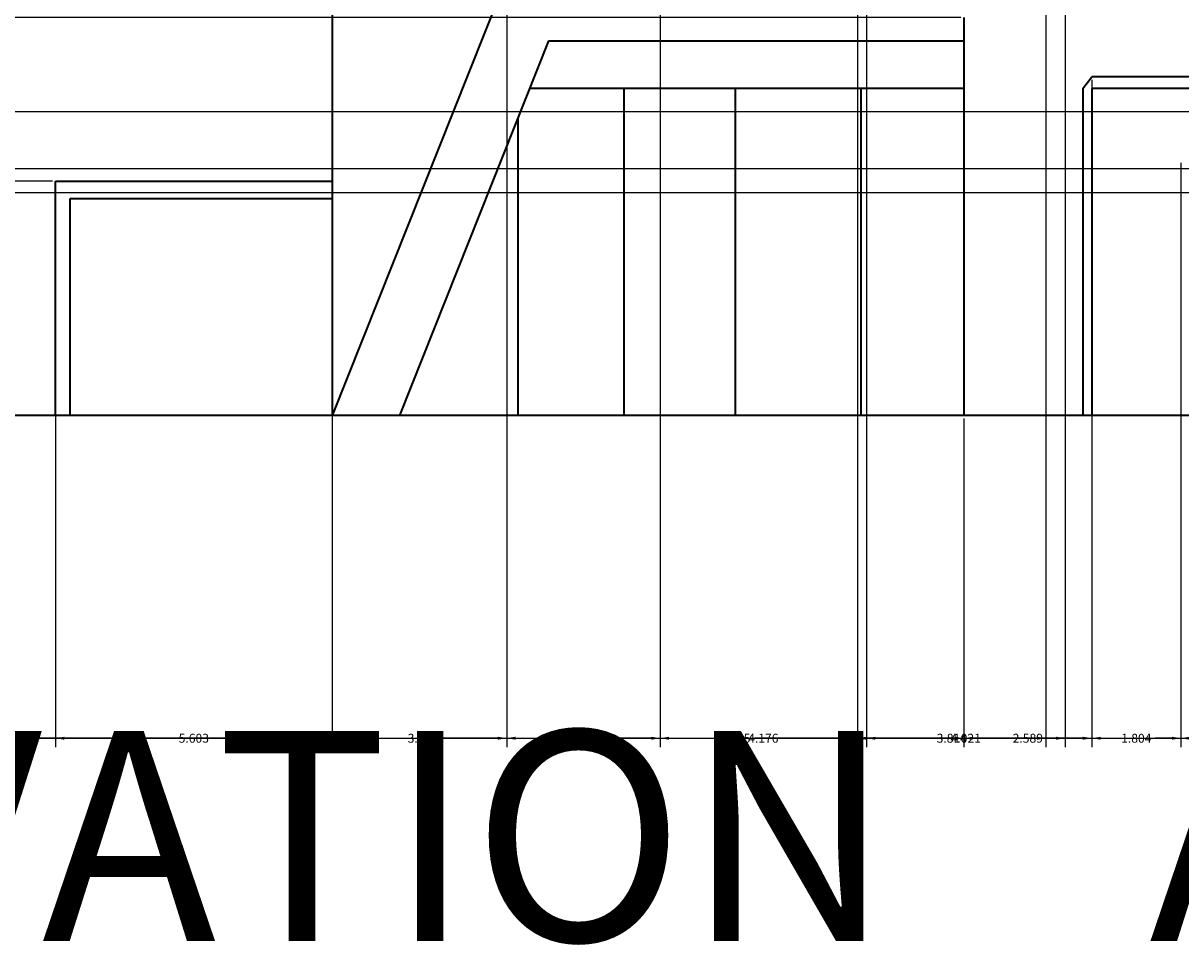
# Model space of a CAD drawing. Units: inches. Extents: x -10 to 130, y -32 to 34.
# Tile 3 of 22: x 25.72 to 49.15, y -32.13 to -13.47. Entities that reach past the tile are written whole.
import ezdxf

# ---------------------------------------------------------------- set-up
doc = ezdxf.new("R2010")
doc.units = ezdxf.units.IN
doc.header["$MEASUREMENT"] = 0
for name, color, linetype, lineweight in [('A-ANNO-DIMS', 2, 'Continuous', 18), ('A-ANNO-TEXT', 7, 'Continuous', 25), ('A-ELEV', 7, 'Continuous', 35)]:
    doc.layers.add(name, color=color, linetype=linetype, lineweight=lineweight)
doc.styles.get("Standard").update_dxf_attribs({"font": 'arial.ttf'})
doc.dimstyles.get("Standard").update_dxf_attribs({"dimtxt": 0.18, "dimasz": 0.18, "dimexe": 0.18, "dimexo": 0.0625, "dimgap": 0.09, "dimtad": 0, "dimtih": 1, "dimtoh": 1, "dimdec": 4, "dimzin": 0, "dimdsep": 46, "dimtxsty": 'Standard', "dimcen": 0.09, "dimadec": 0, "dimazin": 0, "dimtfac": 1, "dimtdec": 4, "dimtofl": 0, "dimtmove": 0, "dimatfit": 3, "dimfxl": 1, "dimtolj": 1, "dimtzin": 0, "dimarcsym": 0})

# ---------------------------------------------------------------- blocks, each defined once
blk = doc.blocks.new('*D1')
at = {"layer": 'A-ANNO-DIMS', "color": 0, "lineweight": -2, "transparency": 16777216}
for p, q in [((5.634, -13.647), (5.634, -28.129)), ((107.933, -21.477), (107.933, -28.129)), ((5.814, -27.949), (56.398, -27.949)), ((107.753, -27.949), (57.169, -27.949))]:
    blk.add_line(p, q, dxfattribs=at)
at = {"layer": 'A-ANNO-DIMS', "color": 0, "transparency": 16777216}
for points in [[(5.814, -27.919), (5.814, -27.979), (5.634, -27.949)], [(107.753, -27.919), (107.753, -27.979), (107.933, -27.949)]]:
    blk.add_solid(points, dxfattribs=at)
at = {"layer": 'Defpoints', "color": 0, "transparency": 16777216}
for p in [(5.634, -13.584), (107.933, -21.414), (107.933, -27.949)]:
    blk.add_point(p, dxfattribs=at)
at = {"layer": 'A-ANNO-DIMS', "color": 0, "transparency": 16777216, "insert": (56.784, -27.949), "char_height": 0.18, "attachment_point": 5}
blk.add_mtext('\\A1;102.3', dxfattribs=at)
blk = doc.blocks.new('*D42')
at = {"layer": 'A-ANNO-DIMS', "color": 0, "lineweight": -2, "transparency": 16777216}
for p, q in [((19.055, -21.477), (19.055, -28.129)), ((31.971, -21.477), (31.971, -28.129)), ((19.235, -27.949), (25.058, -27.949)), ((31.791, -27.949), (25.968, -27.949))]:
    blk.add_line(p, q, dxfattribs=at)
at = {"layer": 'A-ANNO-DIMS', "color": 0, "transparency": 16777216}
for points in [[(19.235, -27.919), (19.235, -27.979), (19.055, -27.949)], [(31.791, -27.919), (31.791, -27.979), (31.971, -27.949)]]:
    blk.add_solid(points, dxfattribs=at)
at = {"layer": 'Defpoints', "color": 0, "transparency": 16777216}
for p in [(19.055, -21.414), (31.971, -21.414), (31.971, -27.949)]:
    blk.add_point(p, dxfattribs=at)
at = {"layer": 'A-ANNO-DIMS', "color": 0, "transparency": 16777216, "insert": (25.513, -27.949), "char_height": 0.18, "attachment_point": 5}
blk.add_mtext('\\A1;12.916', dxfattribs=at)
blk = doc.blocks.new('*D43')
at = {"layer": 'A-ANNO-DIMS', "color": 0, "lineweight": -2, "transparency": 16777216}
for p, q in [((35.505, -12.596), (35.505, -28.129)), ((31.971, -21.477), (31.971, -28.129)), ((32.151, -27.949), (33.414, -27.949)), ((35.325, -27.949), (34.062, -27.949))]:
    blk.add_line(p, q, dxfattribs=at)
at = {"layer": 'A-ANNO-DIMS', "color": 0, "transparency": 16777216}
for points in [[(32.151, -27.919), (32.151, -27.979), (31.971, -27.949)], [(35.325, -27.919), (35.325, -27.979), (35.505, -27.949)]]:
    blk.add_solid(points, dxfattribs=at)
at = {"layer": 'Defpoints', "color": 0, "transparency": 16777216}
for p in [(35.505, -12.534), (31.971, -21.414), (35.505, -27.949)]:
    blk.add_point(p, dxfattribs=at)
at = {"layer": 'A-ANNO-DIMS', "color": 0, "transparency": 16777216, "insert": (33.738, -27.949), "char_height": 0.18, "attachment_point": 5}
blk.add_mtext('\\A1;3.53', dxfattribs=at)
blk = doc.blocks.new('*D44')
at = {"layer": 'A-ANNO-DIMS', "color": 0, "lineweight": -2, "transparency": 16777216}
for p, q in [((35.505, -12.596), (35.505, -28.129)), ((44.76, -21.477), (44.76, -28.129)), ((35.685, -27.949), (39.738, -27.949)), ((44.58, -27.949), (40.527, -27.949))]:
    blk.add_line(p, q, dxfattribs=at)
at = {"layer": 'A-ANNO-DIMS', "color": 0, "transparency": 16777216}
for points in [[(35.685, -27.919), (35.685, -27.979), (35.505, -27.949)], [(44.58, -27.919), (44.58, -27.979), (44.76, -27.949)]]:
    blk.add_solid(points, dxfattribs=at)
at = {"layer": 'Defpoints', "color": 0, "transparency": 16777216}
for p in [(35.505, -12.534), (44.76, -21.414), (44.76, -27.949)]:
    blk.add_point(p, dxfattribs=at)
at = {"layer": 'A-ANNO-DIMS', "color": 0, "transparency": 16777216, "insert": (40.132, -27.949), "char_height": 0.18, "attachment_point": 5}
blk.add_mtext('\\A1;9.255', dxfattribs=at)
blk = doc.blocks.new('*D47')
at = {"layer": 'A-ANNO-DIMS', "color": 0, "lineweight": -2, "transparency": 16777216}
for p, q in [((35.567, -12.534), (129.508, -12.534)), ((129.328, -12.714), (129.328, -16.792)), ((129.328, -21.234), (129.328, -17.156)), ((32.034, -21.414), (129.508, -21.414))]:
    blk.add_line(p, q, dxfattribs=at)
at = {"layer": 'A-ANNO-DIMS', "color": 0, "transparency": 16777216}
for points in [[(129.298, -12.714), (129.358, -12.714), (129.328, -12.534)], [(129.298, -21.234), (129.358, -21.234), (129.328, -21.414)]]:
    blk.add_solid(points, dxfattribs=at)
at = {"layer": 'Defpoints', "color": 0, "transparency": 16777216}
for p in [(35.505, -12.534), (31.971, -21.414), (129.328, -21.414)]:
    blk.add_point(p, dxfattribs=at)
at = {"layer": 'A-ANNO-DIMS', "color": 0, "transparency": 16777216, "insert": (129.328, -16.974), "char_height": 0.18, "attachment_point": 5}
blk.add_mtext('\\A1;8.88', dxfattribs=at)
blk = doc.blocks.new('*D49')
at = {"layer": 'A-ANNO-DIMS', "color": 0, "lineweight": -2, "transparency": 16777216}
for p, q in [((44.697, -13.356), (-9.564, -13.356)), ((-9.384, -13.536), (-9.384, -17.203)), ((-9.384, -21.234), (-9.384, -17.567)), ((44.697, -21.414), (-9.564, -21.414))]:
    blk.add_line(p, q, dxfattribs=at)
at = {"layer": 'A-ANNO-DIMS', "color": 0, "transparency": 16777216}
for points in [[(-9.414, -13.536), (-9.354, -13.536), (-9.384, -13.356)], [(-9.414, -21.234), (-9.354, -21.234), (-9.384, -21.414)]]:
    blk.add_solid(points, dxfattribs=at)
at = {"layer": 'Defpoints', "color": 0, "transparency": 16777216}
for p in [(44.76, -13.356), (-9.384, -21.414), (44.76, -21.414)]:
    blk.add_point(p, dxfattribs=at)
at = {"layer": 'A-ANNO-DIMS', "color": 0, "transparency": 16777216, "insert": (-9.384, -17.385), "char_height": 0.18, "attachment_point": 5}
blk.add_mtext('\\A1;8.059', dxfattribs=at)
blk = doc.blocks.new('*D50')
at = {"layer": 'A-ANNO-DIMS', "color": 0, "lineweight": -2, "transparency": 16777216}
for p, q in [((47.349, -14.617), (47.349, -28.129)), ((44.76, -21.477), (44.76, -28.129)), ((44.94, -27.949), (45.659, -27.949)), ((47.169, -27.949), (46.45, -27.949))]:
    blk.add_line(p, q, dxfattribs=at)
at = {"layer": 'A-ANNO-DIMS', "color": 0, "transparency": 16777216}
for points in [[(44.94, -27.919), (44.94, -27.979), (44.76, -27.949)], [(47.169, -27.919), (47.169, -27.979), (47.349, -27.949)]]:
    blk.add_solid(points, dxfattribs=at)
at = {"layer": 'Defpoints', "color": 0, "transparency": 16777216}
for p in [(47.349, -14.555), (44.76, -21.414), (47.349, -27.949)]:
    blk.add_point(p, dxfattribs=at)
at = {"layer": 'A-ANNO-DIMS', "color": 0, "transparency": 16777216, "insert": (46.055, -27.949), "char_height": 0.18, "attachment_point": 5}
blk.add_mtext('\\A1;2.589', dxfattribs=at)
blk = doc.blocks.new('*D51')
at = {"layer": 'A-ANNO-DIMS', "color": 0, "lineweight": -2, "transparency": 16777216}
for p, q in [((47.349, -14.617), (47.349, -28.129)), ((49.153, -16.297), (49.153, -28.129)), ((47.529, -27.949), (47.866, -27.949)), ((48.973, -27.949), (48.636, -27.949))]:
    blk.add_line(p, q, dxfattribs=at)
at = {"layer": 'A-ANNO-DIMS', "color": 0, "transparency": 16777216}
for points in [[(47.529, -27.919), (47.529, -27.979), (47.349, -27.949)], [(48.973, -27.919), (48.973, -27.979), (49.153, -27.949)]]:
    blk.add_solid(points, dxfattribs=at)
at = {"layer": 'Defpoints', "color": 0, "transparency": 16777216}
for p in [(47.349, -14.555), (49.153, -16.234), (49.153, -27.949)]:
    blk.add_point(p, dxfattribs=at)
at = {"layer": 'A-ANNO-DIMS', "color": 0, "transparency": 16777216, "insert": (48.251, -27.949), "char_height": 0.18, "attachment_point": 5}
blk.add_mtext('\\A1;1.804', dxfattribs=at)
blk = doc.blocks.new('*D52')
at = {"layer": 'A-ANNO-DIMS', "color": 0, "lineweight": -2, "transparency": 16777216}
for p, q in [((49.153, -16.297), (49.153, -28.129)), ((55.165, -17.677), (55.165, -28.129)), ((49.333, -27.949), (51.782, -27.949)), ((54.985, -27.949), (52.536, -27.949))]:
    blk.add_line(p, q, dxfattribs=at)
at = {"layer": 'A-ANNO-DIMS', "color": 0, "transparency": 16777216}
for points in [[(49.333, -27.919), (49.333, -27.979), (49.153, -27.949)], [(54.985, -27.919), (54.985, -27.979), (55.165, -27.949)]]:
    blk.add_solid(points, dxfattribs=at)
at = {"layer": 'Defpoints', "color": 0, "transparency": 16777216}
for p in [(49.153, -16.234), (55.165, -17.615), (55.165, -27.949)]:
    blk.add_point(p, dxfattribs=at)
at = {"layer": 'A-ANNO-DIMS', "color": 0, "transparency": 16777216, "insert": (52.159, -27.949), "char_height": 0.18, "attachment_point": 5}
blk.add_mtext('\\A1;6.011', dxfattribs=at)
blk = doc.blocks.new('*D64')
at = {"layer": 'A-ANNO-DIMS', "color": 0, "lineweight": -2, "transparency": 16777216}
for p, q in [((82.315, -15.264), (-9.564, -15.264)), ((-9.384, -15.444), (-9.384, -15.659)), ((-9.384, -16.237), (-9.384, -16.022)), ((82.315, -16.417), (-9.564, -16.417))]:
    blk.add_line(p, q, dxfattribs=at)
at = {"layer": 'A-ANNO-DIMS', "color": 0, "transparency": 16777216}
for points in [[(-9.414, -15.444), (-9.354, -15.444), (-9.384, -15.264)], [(-9.414, -16.237), (-9.354, -16.237), (-9.384, -16.417)]]:
    blk.add_solid(points, dxfattribs=at)
at = {"layer": 'Defpoints', "color": 0, "transparency": 16777216}
for p in [(82.377, -15.264), (-9.384, -16.417), (82.377, -16.417)]:
    blk.add_point(p, dxfattribs=at)
at = {"layer": 'A-ANNO-DIMS', "color": 0, "transparency": 16777216, "insert": (-9.384, -15.841), "char_height": 0.18, "attachment_point": 5}
blk.add_mtext('\\A1;1.15', dxfattribs=at)
blk = doc.blocks.new('*D65')
at = {"layer": 'A-ANNO-DIMS', "color": 0, "lineweight": -2, "transparency": 16777216}
for p, q in [((82.315, -16.417), (-9.564, -16.417)), ((-9.384, -16.597), (-9.384, -18.734)), ((-9.384, -21.234), (-9.384, -19.097)), ((80.669, -21.414), (-9.564, -21.414))]:
    blk.add_line(p, q, dxfattribs=at)
at = {"layer": 'A-ANNO-DIMS', "color": 0, "transparency": 16777216}
for points in [[(-9.414, -16.597), (-9.354, -16.597), (-9.384, -16.417)], [(-9.414, -21.234), (-9.354, -21.234), (-9.384, -21.414)]]:
    blk.add_solid(points, dxfattribs=at)
at = {"layer": 'Defpoints', "color": 0, "transparency": 16777216}
for p in [(-9.384, -16.417), (82.377, -16.417), (80.731, -21.414)]:
    blk.add_point(p, dxfattribs=at)
at = {"layer": 'A-ANNO-DIMS', "color": 0, "transparency": 16777216, "insert": (-9.384, -18.916), "char_height": 0.18, "attachment_point": 5}
blk.add_mtext('\\A1;4.998', dxfattribs=at)
blk = doc.blocks.new('*D69')
at = {"layer": 'A-ANNO-DIMS', "color": 0, "lineweight": -2, "transparency": 16777216}
for p, q in [((89.095, -16.906), (-9.564, -16.906)), ((-9.384, -17.086), (-9.384, -18.979)), ((-9.384, -21.234), (-9.384, -19.342)), ((89.095, -21.414), (-9.564, -21.414))]:
    blk.add_line(p, q, dxfattribs=at)
at = {"layer": 'A-ANNO-DIMS', "color": 0, "transparency": 16777216}
for points in [[(-9.414, -17.086), (-9.354, -17.086), (-9.384, -16.906)], [(-9.414, -21.234), (-9.354, -21.234), (-9.384, -21.414)]]:
    blk.add_solid(points, dxfattribs=at)
at = {"layer": 'Defpoints', "color": 0, "transparency": 16777216}
for p in [(89.158, -16.906), (-9.384, -21.414), (89.158, -21.414)]:
    blk.add_point(p, dxfattribs=at)
at = {"layer": 'A-ANNO-DIMS', "color": 0, "transparency": 16777216, "insert": (-9.384, -19.16), "char_height": 0.18, "attachment_point": 5}
blk.add_mtext('\\A1;4.508', dxfattribs=at)
blk = doc.blocks.new('*D123')
at = {"layer": 'A-ANNO-DIMS', "color": 0, "lineweight": -2, "transparency": 16777216}
for p, q in [((35.505, -0.476), (35.505, -28.129)), ((38.612, -0.476), (38.612, -28.129)), ((35.685, -27.949), (36.665, -27.949)), ((38.432, -27.949), (37.452, -27.949))]:
    blk.add_line(p, q, dxfattribs=at)
at = {"layer": 'A-ANNO-DIMS', "color": 0, "transparency": 16777216}
for points in [[(35.685, -27.919), (35.685, -27.979), (35.505, -27.949)], [(38.432, -27.919), (38.432, -27.979), (38.612, -27.949)]]:
    blk.add_solid(points, dxfattribs=at)
at = {"layer": 'Defpoints', "color": 0, "transparency": 16777216}
for p in [(35.505, -0.414), (38.612, -0.414), (38.612, -27.949)]:
    blk.add_point(p, dxfattribs=at)
at = {"layer": 'A-ANNO-DIMS', "color": 0, "transparency": 16777216, "insert": (37.058, -27.949), "char_height": 0.18, "attachment_point": 5}
blk.add_mtext('\\A1;3.108', dxfattribs=at)
blk = doc.blocks.new('*D124')
at = {"layer": 'A-ANNO-DIMS', "color": 0, "lineweight": -2, "transparency": 16777216}
for p, q in [((38.612, -7.112), (38.612, -28.129)), ((42.788, -7.112), (42.788, -28.129)), ((38.792, -27.949), (40.303, -27.949)), ((42.608, -27.949), (41.097, -27.949))]:
    blk.add_line(p, q, dxfattribs=at)
at = {"layer": 'A-ANNO-DIMS', "color": 0, "transparency": 16777216}
for points in [[(38.792, -27.919), (38.792, -27.979), (38.612, -27.949)], [(42.608, -27.919), (42.608, -27.979), (42.788, -27.949)]]:
    blk.add_solid(points, dxfattribs=at)
at = {"layer": 'Defpoints', "color": 0, "transparency": 16777216}
for p in [(38.612, -7.05), (42.788, -7.05), (42.788, -27.949)]:
    blk.add_point(p, dxfattribs=at)
at = {"layer": 'A-ANNO-DIMS', "color": 0, "transparency": 16777216, "insert": (40.7, -27.949), "char_height": 0.18, "attachment_point": 5}
blk.add_mtext('\\A1;4.176', dxfattribs=at)
blk = doc.blocks.new('*D126')
at = {"layer": 'A-ANNO-DIMS', "color": 0, "lineweight": -2, "transparency": 16777216}
for p, q in [((42.609, -3.206), (42.609, -28.129)), ((46.423, -3.206), (46.423, -28.129)), ((42.789, -27.949), (44.123, -27.949)), ((46.243, -27.949), (44.909, -27.949))]:
    blk.add_line(p, q, dxfattribs=at)
at = {"layer": 'A-ANNO-DIMS', "color": 0, "transparency": 16777216}
for points in [[(42.789, -27.919), (42.789, -27.979), (42.609, -27.949)], [(46.243, -27.919), (46.243, -27.979), (46.423, -27.949)]]:
    blk.add_solid(points, dxfattribs=at)
at = {"layer": 'Defpoints', "color": 0, "transparency": 16777216}
for p in [(42.609, -3.144), (46.423, -3.144), (46.423, -27.949)]:
    blk.add_point(p, dxfattribs=at)
at = {"layer": 'A-ANNO-DIMS', "color": 0, "transparency": 16777216, "insert": (44.516, -27.949), "char_height": 0.18, "attachment_point": 5}
blk.add_mtext('\\A1;3.814', dxfattribs=at)
blk = doc.blocks.new('*D128')
at = {"layer": 'A-ANNO-DIMS', "color": 0, "lineweight": -2, "transparency": 16777216}
for p, q in [((42.788, -8.923), (42.788, -28.129)), ((46.809, -8.923), (46.809, -28.129)), ((42.968, -27.949), (44.419, -27.949)), ((46.629, -27.949), (45.178, -27.949))]:
    blk.add_line(p, q, dxfattribs=at)
at = {"layer": 'A-ANNO-DIMS', "color": 0, "transparency": 16777216}
for points in [[(42.968, -27.919), (42.968, -27.979), (42.788, -27.949)], [(46.629, -27.919), (46.629, -27.979), (46.809, -27.949)]]:
    blk.add_solid(points, dxfattribs=at)
at = {"layer": 'Defpoints', "color": 0, "transparency": 16777216}
for p in [(42.788, -8.861), (46.809, -8.861), (46.809, -27.949)]:
    blk.add_point(p, dxfattribs=at)
at = {"layer": 'A-ANNO-DIMS', "color": 0, "transparency": 16777216, "insert": (44.798, -27.949), "char_height": 0.18, "attachment_point": 5}
blk.add_mtext('\\A1;4.021', dxfattribs=at)
blk = doc.blocks.new('*D134')
at = {"layer": 'A-ANNO-DIMS', "color": 0, "lineweight": -2, "transparency": 16777216}
for p, q in [((26.368, -16.731), (26.368, -28.129)), ((31.971, -16.731), (31.971, -28.129)), ((26.548, -27.949), (28.776, -27.949)), ((31.791, -27.949), (29.563, -27.949))]:
    blk.add_line(p, q, dxfattribs=at)
at = {"layer": 'A-ANNO-DIMS', "color": 0, "transparency": 16777216}
for points in [[(26.548, -27.919), (26.548, -27.979), (26.368, -27.949)], [(31.791, -27.919), (31.791, -27.979), (31.971, -27.949)]]:
    blk.add_solid(points, dxfattribs=at)
at = {"layer": 'Defpoints', "color": 0, "transparency": 16777216}
for p in [(26.368, -16.668), (31.971, -16.668), (31.971, -27.949)]:
    blk.add_point(p, dxfattribs=at)
at = {"layer": 'A-ANNO-DIMS', "color": 0, "transparency": 16777216, "insert": (29.17, -27.949), "char_height": 0.18, "attachment_point": 5}
blk.add_mtext('\\A1;5.603', dxfattribs=at)
blk = doc.blocks.new('*D135')
at = {"layer": 'A-ANNO-DIMS', "color": 0, "lineweight": -2, "transparency": 16777216}
for p, q in [((26.306, -16.668), (-9.564, -16.668)), ((-9.384, -16.848), (-9.384, -18.859)), ((-9.384, -21.234), (-9.384, -19.223)), ((26.306, -21.414), (-9.564, -21.414))]:
    blk.add_line(p, q, dxfattribs=at)
at = {"layer": 'A-ANNO-DIMS', "color": 0, "transparency": 16777216}
for points in [[(-9.414, -16.848), (-9.354, -16.848), (-9.384, -16.668)], [(-9.414, -21.234), (-9.354, -21.234), (-9.384, -21.414)]]:
    blk.add_solid(points, dxfattribs=at)
at = {"layer": 'Defpoints', "color": 0, "transparency": 16777216}
for p in [(26.368, -16.668), (-9.384, -21.414), (26.368, -21.414)]:
    blk.add_point(p, dxfattribs=at)
at = {"layer": 'A-ANNO-DIMS', "color": 0, "transparency": 16777216, "insert": (-9.384, -19.041), "char_height": 0.18, "attachment_point": 5}
blk.add_mtext('\\A1;4.746', dxfattribs=at)

msp = doc.modelspace()

# ---------------------------------------------------------------- linework, layer by layer
at = {"layer": 'A-ELEV'}
for p, q in [((31.9712, -6.2218), (31.9712, -16.1883)), ((35.5046, -12.5339), (31.9712, -21.4145)), ((44.76, -13.3558), (44.76, -21.4145)), ((36.3513, -13.8305), (33.3337, -21.4145)), ((36.3513, -13.8305), (39.4589, -13.8305)), ((39.4589, -13.8305), (44.76, -13.8305)), ((47.1708, -14.7925), (47.3492, -14.555)), ((54.1471, -14.555), (47.3492, -14.555)), ((35.9714, -14.7852), (39.4589, -14.7852)), ((37.874, -14.7852), (37.874, -21.4145)), ((39.4589, -14.7852), (44.76, -14.7852)), ((40.1317, -14.7852), (40.1317, -21.4145)), ((42.6716, -14.7852), (42.6716, -21.4145)), ((47.1708, -14.7925), (47.1708, -21.4145)), ((47.3492, -14.7925), (47.3492, -21.4145)), ((54.1471, -14.7925), (47.3492, -14.7925)), ((35.7292, -15.3939), (35.7292, -21.4145)), ((31.9712, -16.1883), (31.9712, -21.4145)), ((26.3683, -21.4145), (26.3683, -16.668)), ((26.3683, -16.668), (31.9712, -16.668)), ((26.6647, -17.0179), (31.9712, -17.0179)), ((26.6647, -21.4145), (26.6647, -17.0179)), ((31.9712, -21.4145), (21.1687, -21.4145)), ((44.76, -21.4145), (31.9712, -21.4145)), ((55.1648, -21.4145), (44.76, -21.4145))]:
    msp.add_line(p, q, dxfattribs=at)

# ---------------------------------------------------------------- texts
at = {"layer": 'A-ANNO-TEXT'}
msp.add_text('REAR   ELEVATION    AND   LOGISTICS   HUB', height=4.256275, dxfattribs=at).set_placement((-5.4651, -32.0569))

# ---------------------------------------------------------------- dimensions: what is measured, and where the dimension line sits
at = {"layer": 'A-ANNO-DIMS'}
for base, p1, p2, override, picture, middle in [((38.6123, -27.9493), (35.5046, -0.4138), (38.6123, -0.4138), {"dimdec": 3, "dimlfac": 1, "dimrnd": 0, "dimzin": 0, "dimdsep": 46, "dimlunit": 2}, '*D123', (37.0585, -27.9493)), ((46.4227, -27.9493), (42.6089, -3.1438), (46.4227, -3.1438), {"dimdec": 3, "dimlfac": 1, "dimrnd": 0, "dimzin": 0, "dimdsep": 46, "dimlunit": 2}, '*D126', (44.5158, -27.9493)), ((42.7881, -27.9493), (38.6123, -7.05), (42.7881, -7.05), {"dimdec": 3, "dimlfac": 1, "dimrnd": 0, "dimzin": 0, "dimdsep": 46, "dimlunit": 2}, '*D124', (40.7002, -27.9493)), ((46.8089, -27.9493), (42.7881, -8.8608), (46.8089, -8.8608), {"dimdec": 3, "dimlfac": 1, "dimrnd": 0, "dimzin": 0, "dimdsep": 46, "dimlunit": 2}, '*D128', (44.7985, -27.9493)), ((35.5046, -27.9493), (31.9712, -21.4145), (35.5046, -12.5339), {"dimdec": 2, "dimlfac": 1, "dimrnd": 0, "dimzin": 0, "dimdsep": 46, "dimlunit": 2}, '*D43', (33.7379, -27.9493)), ((44.76, -27.9493), (35.5046, -12.5339), (44.76, -21.4145), {"dimdec": 3, "dimlfac": 1, "dimrnd": 0, "dimzin": 0, "dimdsep": 46, "dimlunit": 2}, '*D44', (40.1323, -27.9493)), ((107.9333, -27.9493), (5.634, -13.5841), (107.9333, -21.4145), {"dimdec": 1, "dimlfac": 1, "dimrnd": 0, "dimzin": 0, "dimdsep": 46, "dimlunit": 2}, '*D1', (56.7837, -27.9493)), ((47.3492, -27.9493), (44.76, -21.4145), (47.3492, -14.555), {"dimdec": 3, "dimlfac": 1, "dimrnd": 0, "dimzin": 0, "dimdsep": 46, "dimlunit": 2}, '*D50', (46.0546, -27.9493)), ((49.1533, -27.9493), (47.3492, -14.555), (49.1533, -16.2341), {"dimdec": 3, "dimlfac": 1, "dimrnd": 0, "dimzin": 0, "dimdsep": 46, "dimlunit": 2}, '*D51', (48.2512, -27.9493)), ((55.16483, -27.949305), (49.153331, -16.234138), (55.16483, -17.614631), {"dimdec": 3, "dimlfac": 1, "dimrnd": 0, "dimzin": 0, "dimdsep": 46, "dimlunit": 2}, '*D52', (52.159081, -27.949305)), ((31.9712, -27.9493), (26.3683, -16.668), (31.9712, -16.668), {"dimdec": 3, "dimlfac": 1, "dimrnd": 0, "dimzin": 0, "dimdsep": 46, "dimlunit": 2}, '*D134', (29.1697, -27.9493)), ((31.9712, -27.9493), (19.055, -21.4145), (31.9712, -21.4145), {"dimdec": 3, "dimlfac": 1, "dimrnd": 0, "dimzin": 0, "dimdsep": 46, "dimlunit": 2}, '*D42', (25.5131, -27.9493))]:
    dim = msp.add_linear_dim(base=base, p1=p1, p2=p2, dimstyle='Standard', override=override, dxfattribs=at)
    dim.commit()
    dim.dimension.update_dxf_attribs({"geometry": picture, "text_midpoint": middle})
for base, p1, p2, override, picture, middle in [((129.3277, -21.4145), (35.5046, -12.5339), (31.9712, -21.4145), {"dimdec": 2, "dimlfac": 1, "dimrnd": 0, "dimzin": 0, "dimdsep": 46, "dimlunit": 2}, '*D47', (129.3277, -16.9742)), ((-9.3836, -21.4145), (44.76, -13.3558), (44.76, -21.4145), {"dimdec": 3, "dimlfac": 1, "dimrnd": 0, "dimzin": 0, "dimdsep": 46, "dimlunit": 2}, '*D49', (-9.3836, -17.3852)), ((-9.3836, -16.4166), (82.377, -15.2645), (82.377, -16.4166), {"dimdec": 2, "dimlfac": 1, "dimrnd": 0, "dimzin": 0, "dimdsep": 46, "dimlunit": 2}, '*D64', (-9.3836, -15.8406)), ((-9.3836, -16.4166), (80.7314, -21.4145), (82.377, -16.4166), {"dimdec": 3, "dimlfac": 1, "dimrnd": 0, "dimzin": 0, "dimdsep": 46, "dimlunit": 2}, '*D65', (-9.3836, -18.9156)), ((-9.38355, -21.41449), (26.36827, -16.66804), (26.36827, -21.41449), {"dimdec": 3, "dimlfac": 1, "dimrnd": 0, "dimzin": 0, "dimdsep": 46, "dimlunit": 2}, '*D135', (-9.38355, -19.04127)), ((-9.3836, -21.4145), (89.1578, -16.9063), (89.1578, -21.4145), {"dimdec": 3, "dimlfac": 1, "dimrnd": 0, "dimzin": 0, "dimdsep": 46, "dimlunit": 2}, '*D69', (-9.3836, -19.1604))]:
    dim = msp.add_linear_dim(base=base, p1=p1, p2=p2, angle=90, dimstyle='Standard', override=override, dxfattribs=at)
    dim.commit()
    dim.dimension.update_dxf_attribs({"geometry": picture, "text_midpoint": middle})

doc.saveas('drawing.dxf')
